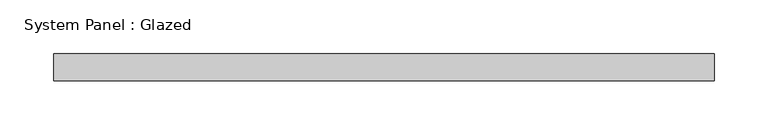
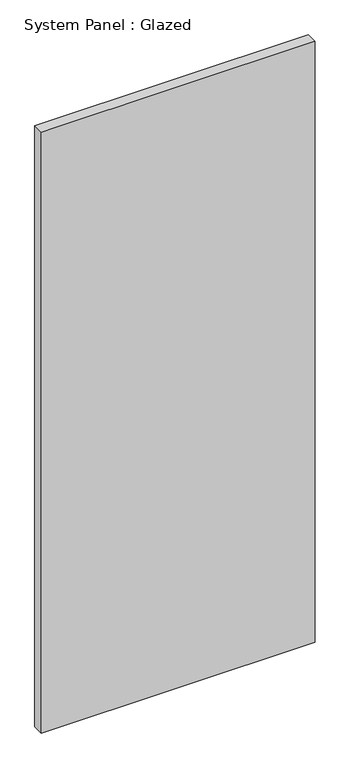
"""IFC4 building model written with IfcOpenShell, lengths in millimetres: plate geometry, System Panel : Glazed."""

from ifc_helpers import new_model, si_unit, origin, origin_with_axes, place, context, project, spatial, polyline, outline, extrude, source, transform, mapped, element, save


def system_panel_glazed_28bcf516(model_context):
    return source(origin(), model_context, "Body", "SweptSolid", [
        extrude(outline(polyline([(307.975, 19.05), (-307.975, 19.05), (-307.975, 44.45), (307.975, 44.45), (307.975, 19.05)])), origin_with_axes(), (0.0, 0.0, 1.0), 1429.4785779),
    ])


if __name__ == "__main__":
    model = new_model("IFC4")
    model_context = context("Model", 3, world=origin())
    ifc_project = project(units=[si_unit("LENGTHUNIT", "METRE", prefix="MILLI")], contexts=[model_context])
    site = spatial("IfcSite", under=ifc_project)
    building = spatial("IfcBuilding", under=site)
    placement = place(None, origin())
    system_panel_glazed_shape = system_panel_glazed_28bcf516(model_context)
    element("IfcPlate", 1, ObjectType="System Panel : Glazed", at=placement, inside=building, context=model_context, shape_type="MappedRepresentation", body=[
        mapped(system_panel_glazed_shape, transform((0.0, 0.0, 0.0), x_axis=(1.0, 0.0, 0.0), y_axis=(0.0, 1.0, 0.0), z_axis=(0.0, 0.0, 1.0))),
    ])
    save(model, "model.ifc")

# Revit data of these elements
# Type "System Panel : Glazed"
#   Construction Type Id = "GSP4R"
#   Analytic Construction = "1/8 in Pilkington single glazing"
#   Visual Light Transmittance = 0.9
#   Solar Heat Gain Coefficient = 0.86
#   Heat Transfer Coefficient (U) = 1.18115 BTU/(h·ft²·°F)
#   Define Thermal Properties by = 1
# Element 1 (IfcPlate, "System Panel : Glazed")
#   Materials on its faces: "Glass"
# Materials
#   "Glass": class "Glass", colour RGB 0 128 192, transparency 0.75, Description = "Soda Lime Glass", Cost = 0
